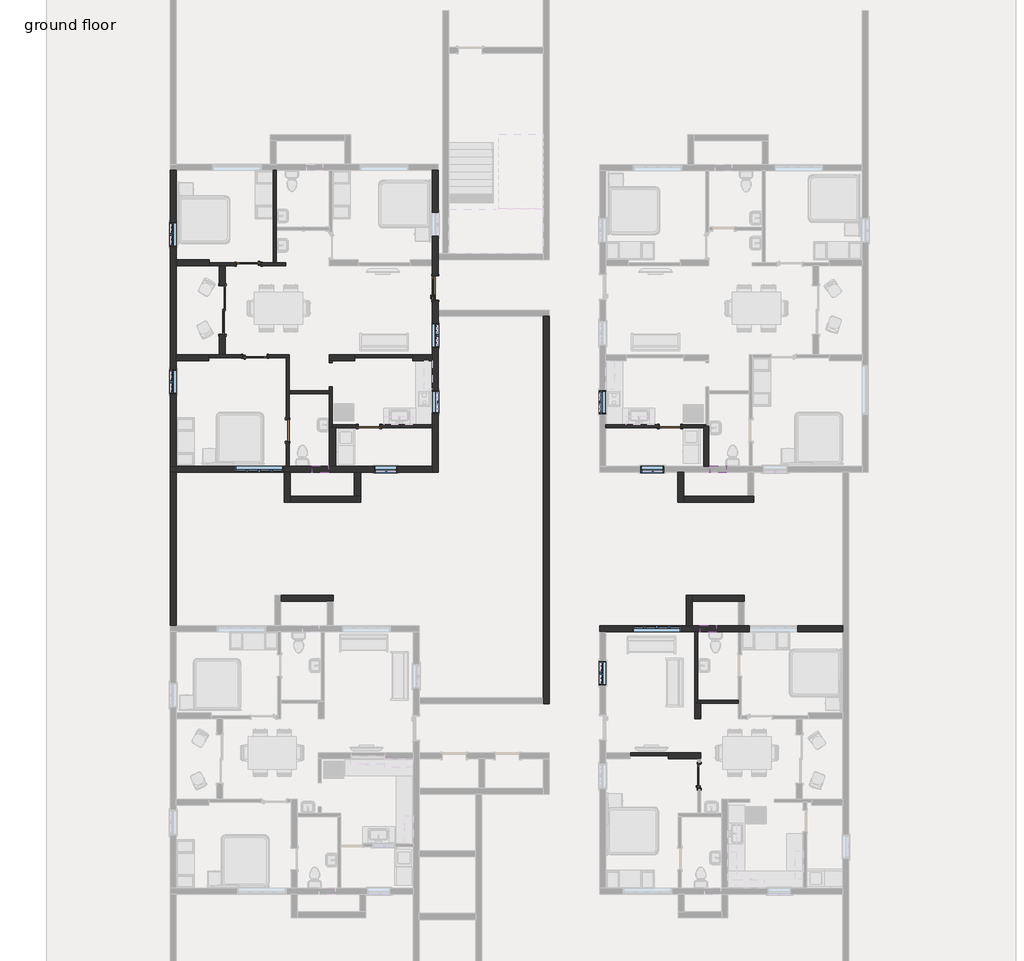
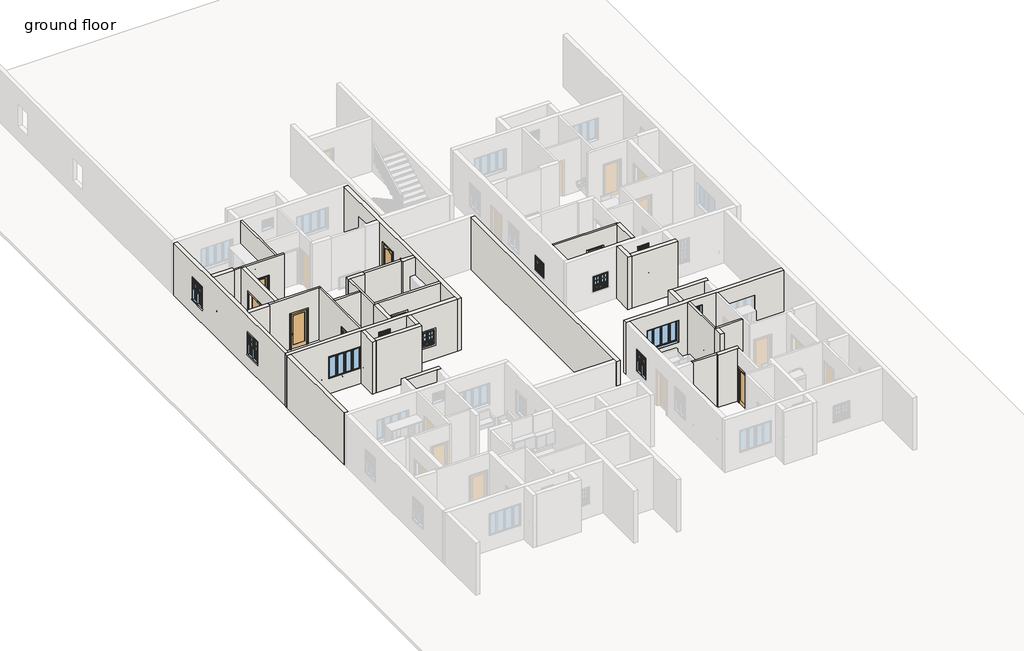
# One storey, part 6 of 16: 36 walls, 13 windows, 8 doors.
"""IFC4 building model written with IfcOpenShell, lengths in millimetres."""

from ifc_helpers import new_model, si_unit, point, frame, origin, place, context, project, spatial, polyline, ellipse_curve, trimmed, outline, extrude, faceted_brep, transform, mapped, element, save
from ifc_brep_helpers import plane_surface, extruded_surface, advanced_brep
from components import door_fe8ae985, door_d4d75d1e, door_a3feeac7, door_3c6ab76a, door_38851409, door_d141acb4, window_ced37e8f, window_5487fb6d, window_f2d8fef0, window_45970670

model = new_model("IFC4")

# Units and contexts
model_context = context("Model", 3, world=origin())
ifc_project = project(units=[si_unit("LENGTHUNIT", "METRE", prefix="MILLI")], contexts=[model_context])

# Site, building, storey
site = spatial("IfcSite", under=ifc_project)
building = spatial("IfcBuilding", under=site)
storey = spatial("IfcBuildingStorey", under=building, Name="ground floor", Elevation=609.6)

# Doors
placement = place(None, origin())
door_shape = door_fe8ae985(model_context)
element("IfcDoor", 1, ObjectType="36\" x 84\"", at=placement, inside=storey, context=model_context, shape_type="MappedRepresentation", body=[
    mapped(door_shape, transform((53146.051243, 27978.3344264, 609.6), x_axis=(0.0, -1.0, 0.0), y_axis=(1.0, 0.0, 0.0), z_axis=(0.0, 0.0, 1.0))),
])
door_2_shape = door_d4d75d1e(model_context)
element("IfcDoor", 2, ObjectType="Door-Double-Sliding : 72\" x 84\"", at=placement, inside=storey, context=model_context, shape_type="MappedRepresentation", body=[
    mapped(door_2_shape, transform((44983.126243, 27148.9150652, 609.6), x_axis=(0.0, -1.0, 0.0), y_axis=(1.0, 0.0, 0.0), z_axis=(0.0, 0.0, 1.0))),
])
door_3_shape = door_a3feeac7(model_context)
element("IfcDoor", 3, ObjectType="Door-Interior-Single-1_Panel-Wood : 36\" x 84\"", at=placement, inside=storey, context=model_context, shape_type="MappedRepresentation", body=[
    mapped(door_3_shape, transform((46097.551243, 28879.2900652, 609.6), x_axis=(-1.0, 0.0, 0.0), y_axis=(0.0, -1.0, 0.0), z_axis=(0.0, 0.0, 1.0))),
])
element("IfcDoor", 4, ObjectType="Door-Interior-Single-1_Panel-Wood : 36\" x 84\"", at=placement, inside=storey, context=model_context, shape_type="MappedRepresentation", body=[
    mapped(door_3_shape, transform((46338.851243, 25405.8400652, 609.6), x_axis=(1.0, 0.0, 0.0), y_axis=(0.0, 1.0, 0.0), z_axis=(0.0, 0.0, 1.0))),
])
door_4_shape = door_3c6ab76a(model_context)
element("IfcDoor", 5, ObjectType="Door-Interior-Single-1_Panel-Wood : 36\" x 84\"", at=placement, inside=storey, context=model_context, shape_type="MappedRepresentation", body=[
    mapped(door_4_shape, transform((63106.2062819, 9553.0650652, 609.6), x_axis=(0.0, 1.0, 0.0), y_axis=(-1.0, 0.0, 0.0), z_axis=(0.0, 0.0, 1.0))),
])
door_5_shape = door_38851409(model_context)
element("IfcDoor", 6, ObjectType="Single-Flush : 32\" x 84\"", at=placement, inside=storey, context=model_context, shape_type="MappedRepresentation", body=[
    mapped(door_5_shape, transform((47567.576243, 22592.7211333, 609.6), x_axis=(0.0, 1.0, 0.0), y_axis=(-1.0, 0.0, 0.0), z_axis=(0.0, 0.0, 1.0))),
])
element("IfcDoor", 7, ObjectType="Single-Flush : 32\" x 84\"", at=placement, inside=storey, context=model_context, shape_type="MappedRepresentation", body=[
    mapped(door_5_shape, transform((61998.1312819, 22754.7150652, 609.6), x_axis=(1.0, 0.0, 0.0), y_axis=(0.0, 1.0, 0.0), z_axis=(0.0, 0.0, 1.0))),
])
door_6_shape = door_d141acb4(model_context)
element("IfcDoor", 8, ObjectType="Single-Flush : 32\" x 84\"", at=placement, inside=storey, context=model_context, shape_type="MappedRepresentation", body=[
    mapped(door_6_shape, transform((50634.626243, 22754.7150652, 609.6), x_axis=(-1.0, 0.0, 0.0), y_axis=(0.0, -1.0, 0.0), z_axis=(0.0, 0.0, 1.0))),
])

# Walls
element("IfcWall", 9, ObjectType="Generic - 4.5\"", at=placement, inside=storey, context=model_context, shape_type="Brep", body=[
    faceted_brep([(62404.5312819, 22697.5650652, 2743.2), (62404.5312819, 22697.5650652, 609.6), (63268.1312819, 22697.5650652, 609.6), (63268.1312819, 22697.5650652, 3810.0), (59585.1312819, 22697.5650652, 3810.0), (59585.1312819, 22697.5650652, 609.6), (61591.7312819, 22697.5650652, 609.6), (61591.7312819, 22697.5650652, 2743.2), (63357.0312819, 22811.8650652, 609.6), (62404.5312819, 22811.8650652, 609.6), (62404.5312819, 22811.8650652, 2743.2), (61591.7312819, 22811.8650652, 2743.2), (61591.7312819, 22811.8650652, 609.6), (59585.1312819, 22811.8650652, 609.6), (59585.1312819, 22811.8650652, 3810.0), (63357.0312819, 22811.8650652, 3810.0), (63357.0312819, 22754.7150652, 609.6), (63268.1312819, 22754.7150652, 609.6), (63268.1312819, 22754.7150652, 3810.0), (63357.0312819, 22754.7150652, 3810.0)], [[[0, 1, 2, 3, 4, 5, 6, 7]], [[8, 9, 10, 11, 12, 13, 14, 15]], [[6, 5, 13, 12]], [[2, 1, 9, 8, 16, 17]], [[4, 3, 18, 19, 15, 14]], [[3, 2, 17, 18]], [[17, 16, 19, 18]], [[16, 8, 15, 19]], [[5, 4, 14, 13]], [[10, 9, 1, 0]], [[11, 10, 0, 7]], [[12, 11, 7, 6]]]),
])
element("IfcWall", 10, ObjectType="Generic - 4.5\"", at=placement, inside=storey, context=model_context, shape_type="Brep", body=[
    faceted_brep([(47027.826243, 32412.9272014, 609.6), (47027.826243, 28933.2650652, 609.6), (47027.826243, 28933.2650652, 3810.0), (47027.826243, 32412.9272014, 3810.0), (47142.126243, 32412.9272014, 609.6), (47142.126243, 32412.9272014, 3810.0), (47142.126243, 30266.7650652, 3810.0), (47142.126243, 30152.4650652, 3810.0), (47142.126243, 28933.2650652, 3810.0), (47142.126243, 28933.2650652, 609.6), (47142.126243, 30152.4650652, 609.6), (47142.126243, 30266.7650652, 609.6)], [[[0, 1, 2, 3]], [[4, 5, 6, 7, 8, 9, 10, 11]], [[1, 0, 4, 11, 10, 9]], [[3, 2, 8, 7, 6, 5]], [[0, 3, 5, 4]], [[2, 1, 9, 8]]]),
])
element("IfcWall", 11, ObjectType="Generic - 4.5\"", at=placement, inside=storey, context=model_context, shape_type="Brep", body=[
    faceted_brep([(47027.826243, 32412.9272014, 609.6), (47027.826243, 28933.2650652, 609.6), (47027.826243, 28933.2650652, 3810.0), (47027.826243, 32412.9272014, 3810.0), (47142.126243, 32412.9272014, 609.6), (47142.126243, 32412.9272014, 3810.0), (47142.126243, 30266.7650652, 3810.0), (47142.126243, 30152.4650652, 3810.0), (47142.126243, 28933.2650652, 3810.0), (47142.126243, 28933.2650652, 609.6), (47142.126243, 30152.4650652, 609.6), (47142.126243, 30266.7650652, 609.6)], [[[0, 1, 2, 3]], [[4, 5, 6, 7, 8, 9, 10, 11]], [[1, 0, 4, 11, 10, 9]], [[3, 2, 8, 7, 6, 5]], [[0, 3, 5, 4]], [[2, 1, 9, 8]]]),
])
element("IfcWall", 12, ObjectType="Generic - 4.5\"", at=placement, inside=storey, context=model_context, shape_type="Brep", body=[
    faceted_brep([(47498.5665582, 28818.9650652, 609.6), (47498.5665582, 28818.9650652, 3810.0), (45224.426243, 28818.9650652, 3810.0), (44995.826243, 28818.9650652, 3810.0), (44602.9665582, 28818.9650652, 3810.0), (44602.9665582, 28818.9650652, 609.6), (44995.826243, 28818.9650652, 609.6), (45224.426243, 28818.9650652, 609.6), (45614.951243, 28818.9650652, 609.6), (45614.951243, 28818.9650652, 2768.6), (46580.151243, 28818.9650652, 2768.6), (46580.151243, 28818.9650652, 609.6), (47498.5665582, 28933.2650652, 3810.0), (47498.5665582, 28933.2650652, 609.6), (47142.126243, 28933.2650652, 609.6), (47027.826243, 28933.2650652, 609.6), (46580.151243, 28933.2650652, 609.6), (46580.151243, 28933.2650652, 2768.6), (45614.951243, 28933.2650652, 2768.6), (45614.951243, 28933.2650652, 609.6), (44602.9665582, 28933.2650652, 609.6), (44602.9665582, 28933.2650652, 3810.0), (47027.826243, 28933.2650652, 3810.0), (47142.126243, 28933.2650652, 3810.0)], [[[0, 1, 2, 3, 4, 5, 6, 7, 8, 9, 10, 11]], [[12, 13, 14, 15, 16, 17, 18, 19, 20, 21, 22, 23]], [[13, 0, 11, 16, 15, 14]], [[5, 20, 19, 8, 7, 6]], [[1, 0, 13, 12]], [[4, 3, 2, 1, 12, 23, 22, 21]], [[5, 4, 21, 20]], [[18, 9, 8, 19]], [[9, 18, 17, 10]], [[10, 17, 16, 11]]]),
])
element("IfcWall", 13, ObjectType="Generic - 4.5\"", at=placement, inside=storey, context=model_context, shape_type="Brep", body=[
    faceted_brep([(47624.726243, 25351.8650652, 3810.0), (47510.426243, 25351.8650652, 3810.0), (44588.5228455, 25351.8650652, 3810.0), (44588.5228455, 25351.8650652, 609.6), (45856.251243, 25351.8650652, 609.6), (45856.251243, 25351.8650652, 2768.6), (46821.451243, 25351.8650652, 2768.6), (46821.451243, 25351.8650652, 609.6), (47510.426243, 25351.8650652, 609.6), (47624.726243, 25351.8650652, 609.6), (44588.5228455, 25466.1650652, 3810.0), (44995.826243, 25466.1650652, 3810.0), (45224.426243, 25466.1650652, 3810.0), (47624.726243, 25466.1650652, 3810.0), (47624.726243, 25466.1650652, 609.6), (46821.451243, 25466.1650652, 609.6), (46821.451243, 25466.1650652, 2768.6), (45856.251243, 25466.1650652, 2768.6), (45856.251243, 25466.1650652, 609.6), (45224.426243, 25466.1650652, 609.6), (44995.826243, 25466.1650652, 609.6), (44588.5228455, 25466.1650652, 609.6)], [[[0, 1, 2, 3, 4, 5, 6, 7, 8, 9]], [[10, 11, 12, 13, 14, 15, 16, 17, 18, 19, 20, 21]], [[3, 21, 20, 19, 18, 4]], [[14, 9, 8, 7, 15]], [[2, 1, 0, 13, 12, 11, 10]], [[3, 2, 10, 21]], [[0, 9, 14, 13]], [[6, 16, 15, 7]], [[16, 6, 5, 17]], [[17, 5, 4, 18]]]),
])
element("IfcWall", 14, ObjectType="Generic - 4.5\"", at=placement, inside=storey, context=model_context, shape_type="Brep", body=[
    faceted_brep([(47510.426243, 25351.8650652, 609.6), (47510.426243, 22999.1211333, 609.6), (47510.426243, 22999.1211333, 2743.2), (47510.426243, 22186.3211333, 2743.2), (47510.426243, 22186.3211333, 609.6), (47510.426243, 21249.6272014, 609.6), (47510.426243, 21249.6272014, 3810.0), (47510.426243, 25351.8650652, 3810.0), (47624.726243, 22999.1211333, 2743.2), (47624.726243, 22999.1211333, 609.6), (47624.726243, 23992.9650652, 609.6), (47624.726243, 24107.2650652, 609.6), (47624.726243, 25351.8650652, 609.6), (47624.726243, 25351.8650652, 3810.0), (47624.726243, 24107.2650652, 3810.0), (47624.726243, 23992.9650652, 3810.0), (47624.726243, 21249.6272014, 3810.0), (47624.726243, 21249.6272014, 609.6), (47624.726243, 22186.3211333, 609.6), (47624.726243, 22186.3211333, 2743.2)], [[[0, 1, 2, 3, 4, 5, 6, 7]], [[8, 9, 10, 11, 12, 13, 14, 15, 16, 17, 18, 19]], [[18, 17, 5, 4]], [[12, 11, 10, 9, 1, 0]], [[7, 6, 16, 15, 14, 13]], [[0, 7, 13, 12]], [[6, 5, 17, 16]], [[2, 1, 9, 8]], [[3, 2, 8, 19]], [[4, 3, 19, 18]]]),
])
element("IfcWall", 15, ObjectType="Generic - 4.5\"", at=placement, inside=storey, context=model_context, shape_type="SweptSolid", body=[
    extrude(outline(polyline([(49148.726243, 23992.9650652), (47624.726243, 23992.9650652), (47624.726243, 24107.2650652), (49148.726243, 24107.2650652), (49148.726243, 23992.9650652)])), frame((0.0, 0.0, 609.6), z_axis=(0.0, 0.0, 1.0), x_axis=(1.0, 0.0, 0.0)), (0.0, 0.0, 1.0), 3200.4),
])
element("IfcWall", 16, ObjectType="Generic - 4.5\"", at=placement, inside=storey, context=model_context, shape_type="AdvancedBrep", body=[
    advanced_brep(
    [(49148.726243, 25237.5650652, 609.6), (49148.726243, 25158.1900652, 609.6), (49148.726243, 25158.1900652, 2540.0), (49148.726243, 24243.7900652, 2540.0), (49148.726243, 24243.7900652, 609.6), (49148.726243, 24107.2650652, 609.6), (49148.726243, 23992.9650652, 609.6), (49148.726243, 22697.5650652, 609.6), (49148.726243, 22697.5650652, 3810.0), (49148.726243, 23992.9650652, 3810.0), (49148.726243, 24107.2650652, 3810.0), (49148.726243, 25237.5650652, 3810.0), (49263.026243, 25158.1900652, 2540.0), (49263.026243, 25158.1900652, 609.6), (49263.026243, 25237.5650652, 609.6), (49263.026243, 25237.5650652, 3810.0), (49263.026243, 22811.8650652, 3810.0), (49263.026243, 22697.5650652, 3810.0), (49263.026243, 22697.5650652, 609.6), (49263.026243, 22811.8650652, 609.6), (49263.026243, 24243.7900652, 609.6), (49263.026243, 24243.7900652, 2540.0)],
    [
        (0, 1),
        (1, 2),
        (2, 3, ellipse_curve(frame((49148.726243, 24700.9900652, 2540.0), z_axis=(1.0, 0.0, 0.0), x_axis=(0.0, 1.0, 0.0)), 457.2, 203.2)),
        (3, 4),
        (4, 5),
        (5, 6),
        (6, 7),
        (7, 8),
        (8, 9),
        (9, 10),
        (10, 11),
        (11, 0),
        (12, 13),
        (13, 14),
        (14, 15),
        (15, 16),
        (16, 17),
        (17, 18),
        (18, 19),
        (19, 20),
        (20, 21),
        (21, 12, ellipse_curve(frame((49263.026243, 24700.9900652, 2540.0), z_axis=(-1.0, 0.0, 0.0), x_axis=(0.0, 1.0, 0.0)), 457.2, 203.2)),
        (13, 1),
        (0, 14),
        (18, 7),
        (4, 20),
        (8, 17),
        (15, 11),
        (2, 12),
        (21, 3),
    ],
    [
        plane_surface(frame((49148.726243, 24107.2650652, 609.6), z_axis=(-1.0, 0.0, 0.0), x_axis=(0.0, -1.0, 0.0))),
        plane_surface(frame((49263.026243, 24107.2650652, 609.6), z_axis=(1.0, 0.0, 0.0), x_axis=(0.0, 1.0, 0.0))),
        plane_surface(frame((49148.726243, 25351.8650652, 609.6), z_axis=(0.0, 0.0, -1.0), x_axis=(1.0, 0.0, 0.0))),
        plane_surface(frame((49148.726243, 22754.7150652, 3810.0), z_axis=(0.0, 0.0, 1.0), x_axis=(1.0, 0.0, 0.0))),
        plane_surface(frame((49283.7527857, 22697.5650652, 609.6), z_axis=(0.0, -1.0, 0.0), x_axis=(1.0, 0.0, 0.0))),
        plane_surface(frame((50047.2611034, 25237.5650652, 609.6), z_axis=(0.0, 1.0, 0.0), x_axis=(1.0, 0.0, 0.0))),
        extruded_surface(trimmed(ellipse_curve(frame((49377.326243, 24700.9900652, 2540.0), z_axis=(1.0, 0.0, 0.0), x_axis=(0.0, 1.0, 0.0)), 457.2, 203.2), [point((49377.326243, 25158.1900652, 2540.0))], [point((49377.326243, 24243.7900652, 2540.0))], True, "CARTESIAN"), (-114.30000000000291, 0.0, 0.0), 114.30000000000291),
        plane_surface(frame((49148.726243, 24243.7900652, 2540.0), z_axis=(0.0, 1.0, 0.0), x_axis=(1.0, 0.0, 0.0))),
        plane_surface(frame((49148.726243, 25158.1900652, 609.6), z_axis=(0.0, -1.0, 0.0), x_axis=(1.0, 0.0, 0.0))),
    ],
    [
        (0, [[1, 2, 3, 4, 5, 6, 7, 8, 9, 10, 11, 12]]),
        (1, [[13, 14, 15, 16, 17, 18, 19, 20, 21, 22]]),
        (2, [[-14, 23, -1, 24]]),
        (2, [[-20, -19, 25, -7, -6, -5, 26]]),
        (3, [[-11, -10, -9, 27, -17, -16, 28]]),
        (4, [[-8, -25, -18, -27]]),
        (5, [[-12, -28, -15, -24]]),
        (6, [[-3, 29, -22, 30]]),
        (7, [[-4, -30, -21, -26]]),
        (8, [[-2, -23, -13, -29]]),
    ],
),
])
element("IfcWall", 17, ObjectType="Generic - 4.5\"", at=placement, inside=storey, context=model_context, shape_type="Brep", body=[
    faceted_brep([(49263.026243, 22697.5650652, 609.6), (49377.326243, 22697.5650652, 609.6), (50228.226243, 22697.5650652, 609.6), (50228.226243, 22697.5650652, 2743.2), (51041.026243, 22697.5650652, 2743.2), (51041.026243, 22697.5650652, 609.6), (53034.926243, 22697.5650652, 609.6), (53034.926243, 22697.5650652, 3810.0), (49377.326243, 22697.5650652, 3810.0), (49263.026243, 22697.5650652, 3810.0), (50228.226243, 22811.8650652, 2743.2), (50228.226243, 22811.8650652, 609.6), (49263.026243, 22811.8650652, 609.6), (49263.026243, 22811.8650652, 3810.0), (53034.926243, 22811.8650652, 3810.0), (53034.926243, 22811.8650652, 609.6), (51041.026243, 22811.8650652, 609.6), (51041.026243, 22811.8650652, 2743.2)], [[[0, 1, 2, 3, 4, 5, 6, 7, 8, 9]], [[10, 11, 12, 13, 14, 15, 16, 17]], [[16, 15, 6, 5]], [[12, 11, 2, 1, 0]], [[9, 8, 7, 14, 13]], [[0, 9, 13, 12]], [[7, 6, 15, 14]], [[3, 2, 11, 10]], [[4, 3, 10, 17]], [[5, 4, 17, 16]]]),
])
element("IfcWall", 18, ObjectType="Generic - 4.5\"", at=placement, inside=storey, context=model_context, shape_type="SweptSolid", body=[
    extrude(outline(polyline([(52298.326243, 25351.8650652), (50101.226243, 25351.8650652), (50101.226243, 25466.1650652), (52298.326243, 25466.1650652), (52298.326243, 25351.8650652)])), frame((0.0, 0.0, 609.6), z_axis=(0.0, 0.0, 1.0), x_axis=(1.0, 0.0, 0.0)), (0.0, 0.0, 1.0), 3200.4),
])
element("IfcWall", 19, ObjectType="Generic - 4.5\"", at=placement, inside=storey, context=model_context, shape_type="Brep", body=[
    faceted_brep([(62937.9312819, 15001.3650652, 609.6), (62937.9312819, 12296.2650652, 609.6), (62937.9312819, 12296.2650652, 3810.0), (62937.9312819, 15001.3650652, 3810.0), (63052.2312819, 15001.3650652, 609.6), (63052.2312819, 15001.3650652, 3810.0), (63052.2312819, 12410.5650652, 3810.0), (63052.2312819, 12296.2650652, 3810.0), (63052.2312819, 12296.2650652, 609.6), (63052.2312819, 12410.5650652, 609.6)], [[[0, 1, 2, 3]], [[4, 5, 6, 7, 8, 9]], [[1, 0, 4, 9, 8]], [[3, 2, 7, 6, 5]], [[0, 3, 5, 4]], [[2, 1, 8, 7]]]),
])
element("IfcWall", 20, ObjectType="Generic - 4.5\"", at=placement, inside=storey, context=model_context, shape_type="Brep", body=[
    faceted_brep([(63052.2312819, 12296.2650652, 609.6), (63166.5312819, 12296.2650652, 609.6), (64576.2312819, 12296.2650652, 609.6), (64576.2312819, 12296.2650652, 3810.0), (63166.5312819, 12296.2650652, 3810.0), (63052.2312819, 12296.2650652, 3810.0), (63052.2312819, 12410.5650652, 609.6), (63052.2312819, 12410.5650652, 3810.0), (64576.2312819, 12410.5650652, 3810.0), (64576.2312819, 12410.5650652, 609.6)], [[[0, 1, 2, 3, 4, 5]], [[6, 7, 8, 9]], [[2, 1, 0, 6, 9]], [[5, 4, 3, 8, 7]], [[0, 5, 7, 6]], [[3, 2, 9, 8]]]),
])
element("IfcWall", 21, ObjectType="Generic - 4.5\"", at=placement, inside=storey, context=model_context, shape_type="SweptSolid", body=[
    extrude(outline(polyline([(61941.6438292, 10315.0650652), (60499.5312819, 10315.0650652), (60499.5312819, 10429.3650652), (61941.6438292, 10429.3650652), (61941.6438292, 10315.0650652)])), frame((0.0, 0.0, 609.6), z_axis=(0.0, 0.0, 1.0), x_axis=(1.0, 0.0, 0.0)), (0.0, 0.0, 1.0), 3200.4),
])
element("IfcWall", 22, ObjectType="Generic - 8\"", at=placement, inside=storey, context=model_context, shape_type="Brep", body=[
    faceted_brep([(63471.3312819, 21249.7650652, 609.6), (63471.3312819, 22754.7150652, 609.6), (63471.3312819, 22754.7150652, 3810.0), (63471.3312819, 21249.7650652, 3810.0), (63268.1312819, 21249.7650652, 609.6), (63268.1312819, 21249.7650652, 3810.0), (63268.1312819, 22697.5650652, 3810.0), (63268.1312819, 22754.7150652, 3810.0), (63268.1312819, 22754.7150652, 609.6), (63268.1312819, 22697.5650652, 609.6), (63357.0312819, 22754.7150652, 609.6), (63357.0312819, 22754.7150652, 3810.0)], [[[0, 1, 2, 3]], [[4, 5, 6, 7, 8, 9]], [[1, 0, 4, 9, 8, 10]], [[2, 1, 10, 8, 7, 11]], [[3, 2, 11, 7, 6, 5]], [[0, 3, 5, 4]]]),
])
element("IfcWall", 23, ObjectType="Generic - 9\"", at=placement, inside=storey, context=model_context, shape_type="Brep", body=[
    faceted_brep([(62290.2312819, 21021.1650652, 609.6), (62290.2312819, 19895.3539393, 609.6), (62290.2312819, 19895.3539393, 3810.0), (62290.2312819, 21021.1650652, 3810.0), (62518.8312819, 21021.1650652, 609.6), (62518.8312819, 21021.1650652, 3810.0), (62518.8312819, 20123.9539393, 3810.0), (62518.8312819, 19895.3539393, 3810.0), (62518.8312819, 19895.3539393, 609.6), (62518.8312819, 20123.9539393, 609.6)], [[[0, 1, 2, 3]], [[4, 5, 6, 7, 8, 9]], [[1, 0, 4, 9, 8]], [[3, 2, 7, 6, 5]], [[0, 3, 5, 4]], [[2, 1, 8, 7]]]),
])
element("IfcWall", 24, ObjectType="Generic - 9\"", at=placement, inside=storey, context=model_context, shape_type="Brep", body=[
    faceted_brep([(62518.8312819, 19895.3539393, 609.6), (65172.2983059, 19895.3539393, 609.6), (65172.2983059, 19895.3539393, 3810.0), (62518.8312819, 19895.3539393, 3810.0), (62518.8312819, 20123.9539393, 609.6), (62518.8312819, 20123.9539393, 3810.0), (64943.6983059, 20123.9539393, 3810.0), (65172.2983059, 20123.9539393, 3810.0), (65172.2983059, 20123.9539393, 609.6), (64943.6983059, 20123.9539393, 609.6)], [[[0, 1, 2, 3]], [[4, 5, 6, 7, 8, 9]], [[1, 0, 4, 9, 8]], [[3, 2, 7, 6, 5]], [[0, 3, 5, 4]], [[2, 1, 8, 7]]]),
])
element("IfcWall", 25, ObjectType="Generic - 9\"", at=placement, inside=storey, context=model_context, shape_type="Brep", body=[
    faceted_brep([(53034.926243, 21021.0272014, 3810.0), (53034.926243, 21249.6272014, 3810.0), (53034.926243, 22697.5650652, 3810.0), (53034.926243, 22811.8650652, 3810.0), (53034.926243, 25237.5650652, 3810.0), (53034.926243, 25466.1650652, 3810.0), (53034.926243, 28818.9650652, 3810.0), (53034.926243, 29047.5650652, 3810.0), (53034.926243, 32412.9272014, 3810.0), (53034.926243, 32412.9272014, 609.6), (53034.926243, 29047.5650652, 609.6), (53034.926243, 28818.9650652, 609.6), (53034.926243, 28460.9344264, 609.6), (53034.926243, 28460.9344264, 2768.6), (53034.926243, 27495.7344264, 2768.6), (53034.926243, 27495.7344264, 609.6), (53034.926243, 25466.1650652, 609.6), (53034.926243, 25237.5650652, 609.6), (53034.926243, 22811.8650652, 609.6), (53034.926243, 22697.5650652, 609.6), (53034.926243, 21249.6272014, 609.6), (53034.926243, 21021.0272014, 609.6), (53034.926243, 26644.8344264, 2844.8), (53034.926243, 25730.4344264, 2844.8), (53034.926243, 25730.4344264, 1524.0), (53034.926243, 26644.8344264, 1524.0), (53034.926243, 30838.2650652, 2844.8), (53034.926243, 29923.8650652, 2844.8), (53034.926243, 29923.8650652, 1524.0), (53034.926243, 30838.2650652, 1524.0), (53034.926243, 23240.4900652, 2438.4), (53034.926243, 23240.4900652, 1524.0), (53034.926243, 24104.0900652, 1524.0), (53034.926243, 24104.0900652, 2438.4), (53263.526243, 32412.9272014, 3810.0), (53263.526243, 29276.1650652, 3810.0), (53263.526243, 29047.5650652, 3810.0), (53263.526243, 27137.7037877, 3810.0), (53263.526243, 26909.1037877, 3810.0), (53263.526243, 21021.0272014, 3810.0), (53263.526243, 21021.0272014, 609.6), (53263.526243, 26909.1037877, 609.6), (53263.526243, 27137.7037877, 609.6), (53263.526243, 27495.7344264, 609.6), (53263.526243, 27495.7344264, 2768.6), (53263.526243, 28460.9344264, 2768.6), (53263.526243, 28460.9344264, 609.6), (53263.526243, 29047.5650652, 609.6), (53263.526243, 29276.1650652, 609.6), (53263.526243, 32412.9272014, 609.6), (53263.526243, 26644.8344264, 2844.8), (53263.526243, 26644.8344264, 1524.0), (53263.526243, 25730.4344264, 1524.0), (53263.526243, 25730.4344264, 2844.8), (53263.526243, 30838.2650652, 2844.8), (53263.526243, 30838.2650652, 1524.0), (53263.526243, 29923.8650652, 1524.0), (53263.526243, 29923.8650652, 2844.8), (53263.526243, 23240.4900652, 2438.4), (53263.526243, 24104.0900652, 2438.4), (53263.526243, 24104.0900652, 1524.0), (53263.526243, 23240.4900652, 1524.0)], [[[0, 1, 2, 3, 4, 5, 6, 7, 8, 9, 10, 11, 12, 13, 14, 15, 16, 17, 18, 19, 20, 21], [22, 23, 24, 25], [26, 27, 28, 29], [30, 31, 32, 33]], [[34, 35, 36, 37, 38, 39, 40, 41, 42, 43, 44, 45, 46, 47, 48, 49], [50, 51, 52, 53], [54, 55, 56, 57], [58, 59, 60, 61]], [[9, 49, 48, 47, 46, 12, 11, 10]], [[40, 21, 20, 19, 18, 17, 16, 15, 43, 42, 41]], [[8, 7, 6, 5, 4, 3, 2, 1, 0, 39, 38, 37, 36, 35, 34]], [[9, 8, 34, 49]], [[0, 21, 40, 39]], [[14, 44, 43, 15]], [[44, 14, 13, 45]], [[45, 13, 12, 46]], [[51, 50, 22, 25]], [[52, 51, 25, 24]], [[53, 52, 24, 23]], [[50, 53, 23, 22]], [[55, 54, 26, 29]], [[56, 55, 29, 28]], [[57, 56, 28, 27]], [[54, 57, 27, 26]], [[31, 30, 58, 61]], [[32, 31, 61, 60]], [[33, 32, 60, 59]], [[30, 33, 59, 58]]]),
])
element("IfcWall", 26, ObjectType="Generic - 9\"", at=placement, inside=storey, context=model_context, shape_type="Brep", body=[
    faceted_brep([(53034.926243, 21249.6272014, 609.6), (49377.326243, 21249.6272014, 609.6), (49148.726243, 21249.6272014, 609.6), (47624.726243, 21249.6272014, 609.6), (47510.426243, 21249.6272014, 609.6), (43370.226243, 21249.6272014, 609.6), (43141.626243, 21249.6272014, 609.6), (43141.626243, 21249.6272014, 3810.0), (43370.226243, 21249.6272014, 3810.0), (47510.426243, 21249.6272014, 3810.0), (47624.726243, 21249.6272014, 3810.0), (49148.726243, 21249.6272014, 3810.0), (49377.326243, 21249.6272014, 3810.0), (53034.926243, 21249.6272014, 3810.0), (45580.859219, 21249.6272014, 2870.2), (45580.859219, 21249.6272014, 1524.0), (47409.659219, 21249.6272014, 1524.0), (47409.659219, 21249.6272014, 2870.2), (50843.18, 21249.6272014, 2438.4), (50843.18, 21249.6272014, 1524.0), (51706.78, 21249.6272014, 1524.0), (51706.78, 21249.6272014, 2438.4), (49110.626243, 21249.6272014, 3352.8), (48501.026243, 21249.6272014, 3352.8), (48501.026243, 21249.6272014, 2743.2), (49110.626243, 21249.6272014, 2743.2), (53034.926243, 21021.0272014, 609.6), (53034.926243, 21021.0272014, 3810.0), (50322.48, 21021.0272014, 3810.0), (50093.88, 21021.0272014, 3810.0), (47676.359219, 21021.0272014, 3810.0), (47447.759219, 21021.0272014, 3810.0), (43370.226243, 21021.0272014, 3810.0), (43141.626243, 21021.0272014, 3810.0), (43141.626243, 21021.0272014, 609.6), (43370.226243, 21021.0272014, 609.6), (47447.759219, 21021.0272014, 609.6), (47676.359219, 21021.0272014, 609.6), (50093.88, 21021.0272014, 609.6), (50322.48, 21021.0272014, 609.6), (45580.859219, 21021.0272014, 2870.2), (47409.659219, 21021.0272014, 2870.2), (47409.659219, 21021.0272014, 1524.0), (45580.859219, 21021.0272014, 1524.0), (50843.18, 21021.0272014, 2438.4), (51706.78, 21021.0272014, 2438.4), (51706.78, 21021.0272014, 1524.0), (50843.18, 21021.0272014, 1524.0), (49110.626243, 21021.0272014, 3352.8), (49110.626243, 21021.0272014, 2743.2), (48501.026243, 21021.0272014, 2743.2), (48501.026243, 21021.0272014, 3352.8)], [[[0, 1, 2, 3, 4, 5, 6, 7, 8, 9, 10, 11, 12, 13], [14, 15, 16, 17], [18, 19, 20, 21], [22, 23, 24, 25]], [[26, 27, 28, 29, 30, 31, 32, 33, 34, 35, 36, 37, 38, 39], [40, 41, 42, 43], [44, 45, 46, 47], [48, 49, 50, 51]], [[6, 5, 4, 3, 2, 1, 0, 26, 39, 38, 37, 36, 35, 34]], [[13, 12, 11, 10, 9, 8, 7, 33, 32, 31, 30, 29, 28, 27]], [[0, 13, 27, 26]], [[7, 6, 34, 33]], [[15, 14, 40, 43]], [[16, 15, 43, 42]], [[17, 16, 42, 41]], [[14, 17, 41, 40]], [[19, 18, 44, 47]], [[20, 19, 47, 46]], [[21, 20, 46, 45]], [[18, 21, 45, 44]], [[49, 48, 22, 25]], [[50, 49, 25, 24]], [[51, 50, 24, 23]], [[48, 51, 23, 22]]]),
])
element("IfcWall", 27, ObjectType="Generic - 9\"", at=placement, inside=storey, context=model_context, shape_type="Brep", body=[
    faceted_brep([(43370.226243, 21249.6272014, 609.6), (43370.226243, 25237.5650652, 609.6), (43370.226243, 25466.1650652, 609.6), (43370.226243, 28818.9650652, 609.6), (43370.226243, 29047.5650652, 609.6), (43370.226243, 32412.9272014, 609.6), (43370.226243, 32412.9272014, 3810.0), (43370.226243, 29047.5650652, 3810.0), (43370.226243, 28818.9650652, 3810.0), (43370.226243, 25466.1650652, 3810.0), (43370.226243, 25237.5650652, 3810.0), (43370.226243, 21249.6272014, 3810.0), (43370.226243, 23980.2650652, 2844.8), (43370.226243, 24894.6650652, 2844.8), (43370.226243, 24894.6650652, 1524.0), (43370.226243, 23980.2650652, 1524.0), (43370.226243, 29542.8650652, 2844.8), (43370.226243, 30457.2650652, 2844.8), (43370.226243, 30457.2650652, 1524.0), (43370.226243, 29542.8650652, 1524.0), (43141.626243, 21249.6272014, 609.6), (43141.626243, 21249.6272014, 3810.0), (43141.626243, 32412.9272014, 3810.0), (43141.626243, 32412.9272014, 609.6), (43141.626243, 23980.2650652, 2844.8), (43141.626243, 23980.2650652, 1524.0), (43141.626243, 24894.6650652, 1524.0), (43141.626243, 24894.6650652, 2844.8), (43141.626243, 29542.8650652, 2844.8), (43141.626243, 29542.8650652, 1524.0), (43141.626243, 30457.2650652, 1524.0), (43141.626243, 30457.2650652, 2844.8)], [[[0, 1, 2, 3, 4, 5, 6, 7, 8, 9, 10, 11], [12, 13, 14, 15], [16, 17, 18, 19]], [[20, 21, 22, 23], [24, 25, 26, 27], [28, 29, 30, 31]], [[5, 4, 3, 2, 1, 0, 20, 23]], [[11, 10, 9, 8, 7, 6, 22, 21]], [[0, 11, 21, 20]], [[6, 5, 23, 22]], [[25, 24, 12, 15]], [[26, 25, 15, 14]], [[27, 26, 14, 13]], [[24, 27, 13, 12]], [[29, 28, 16, 19]], [[30, 29, 19, 18]], [[31, 30, 18, 17]], [[28, 31, 17, 16]]]),
])
element("IfcWall", 28, ObjectType="Generic - 9\"", at=placement, inside=storey, context=model_context, shape_type="Brep", body=[
    faceted_brep([(43370.226243, 28818.9650652, 609.6), (44602.9665582, 28818.9650652, 609.6), (44602.9665582, 28818.9650652, 3810.0), (43370.226243, 28818.9650652, 3810.0), (43370.226243, 29047.5650652, 609.6), (43370.226243, 29047.5650652, 3810.0), (44602.9665582, 29047.5650652, 3810.0), (44602.9665582, 29047.5650652, 609.6), (44602.9665582, 28933.2650652, 609.6), (44602.9665582, 28933.2650652, 3810.0)], [[[0, 1, 2, 3]], [[4, 5, 6, 7]], [[1, 0, 4, 7, 8]], [[2, 1, 8, 7, 6, 9]], [[3, 2, 9, 6, 5]], [[0, 3, 5, 4]]]),
])
element("IfcWall", 29, ObjectType="Generic - 9\"", at=placement, inside=storey, context=model_context, shape_type="SweptSolid", body=[
    extrude(outline(polyline([(26234.5150652, 2743.2), (26234.5150652, 609.6), (25466.1650652, 609.6), (25466.1650652, 3810.0), (28818.9650652, 3810.0), (28818.9650652, 609.6), (28063.3150652, 609.6), (28063.3150652, 2743.2), (26234.5150652, 2743.2)])), frame((44995.826243, 0.0, 0.0), z_axis=(1.0, 0.0, 0.0), x_axis=(0.0, 1.0, 0.0)), (0.0, 0.0, 1.0), 228.6),
])
element("IfcWall", 30, ObjectType="Generic - 9\"", at=placement, inside=storey, context=model_context, shape_type="Brep", body=[
    faceted_brep([(43370.226243, 25237.5650652, 609.6), (44588.5228455, 25237.5650652, 609.6), (44588.5228455, 25237.5650652, 3810.0), (43370.226243, 25237.5650652, 3810.0), (43370.226243, 25466.1650652, 609.6), (43370.226243, 25466.1650652, 3810.0), (44588.5228455, 25466.1650652, 3810.0), (44588.5228455, 25466.1650652, 609.6), (44588.5228455, 25351.8650652, 609.6), (44588.5228455, 25351.8650652, 3810.0)], [[[0, 1, 2, 3]], [[4, 5, 6, 7]], [[1, 0, 4, 7, 8]], [[2, 1, 8, 7, 6, 9]], [[3, 2, 9, 6, 5]], [[0, 3, 5, 4]]]),
])
element("IfcWall", 31, ObjectType="Generic - 9\"", at=placement, inside=storey, context=model_context, shape_type="Brep", body=[
    faceted_brep([(49377.326243, 21249.6272014, 609.6), (49377.326243, 22697.5650652, 609.6), (49377.326243, 22697.5650652, 3810.0), (49377.326243, 21249.6272014, 3810.0), (49148.726243, 21249.6272014, 609.6), (49148.726243, 21249.6272014, 3810.0), (49148.726243, 22697.5650652, 3810.0), (49148.726243, 22697.5650652, 609.6), (49263.026243, 22697.5650652, 609.6), (49263.026243, 22697.5650652, 3810.0)], [[[0, 1, 2, 3]], [[4, 5, 6, 7]], [[1, 0, 4, 7, 8]], [[3, 2, 9, 6, 5]], [[0, 3, 5, 4]], [[2, 1, 8, 7, 6, 9]]]),
])
element("IfcWall", 32, ObjectType="Generic - 9\"", at=placement, inside=storey, context=model_context, shape_type="Brep", body=[
    faceted_brep([(53034.926243, 25466.1650652, 609.6), (52298.326243, 25466.1650652, 609.6), (52298.326243, 25466.1650652, 3810.0), (53034.926243, 25466.1650652, 3810.0), (53034.926243, 25237.5650652, 609.6), (53034.926243, 25237.5650652, 3810.0), (52298.326243, 25237.5650652, 3810.0), (52298.326243, 25237.5650652, 609.6), (52298.326243, 25351.8650652, 609.6), (52298.326243, 25351.8650652, 3810.0)], [[[0, 1, 2, 3]], [[4, 5, 6, 7]], [[1, 0, 4, 7, 8]], [[2, 1, 8, 7, 6, 9]], [[3, 2, 9, 6, 5]], [[0, 3, 5, 4]]]),
])
element("IfcWall", 33, ObjectType="Generic - 9\"", at=placement, inside=storey, context=model_context, shape_type="Brep", body=[
    faceted_brep([(50101.226243, 25466.1650652, 609.6), (49148.726243, 25466.1650652, 609.6), (49148.726243, 25466.1650652, 3810.0), (50101.226243, 25466.1650652, 3810.0), (50101.226243, 25237.5650652, 609.6), (50101.226243, 25237.5650652, 3810.0), (49263.026243, 25237.5650652, 3810.0), (49148.726243, 25237.5650652, 3810.0), (49148.726243, 25237.5650652, 609.6), (49263.026243, 25237.5650652, 609.6), (50101.226243, 25351.8650652, 609.6), (50101.226243, 25351.8650652, 3810.0)], [[[0, 1, 2, 3]], [[4, 5, 6, 7, 8, 9]], [[1, 0, 10, 4, 9, 8]], [[3, 2, 7, 6, 5, 11]], [[0, 3, 11, 5, 4, 10]], [[2, 1, 8, 7]]]),
])
element("IfcWall", 34, ObjectType="Generic - 9\"", at=placement, inside=storey, context=model_context, shape_type="Brep", body=[
    faceted_brep([(47447.759219, 21021.0272014, 609.6), (47447.759219, 19895.3539393, 609.6), (47447.759219, 19895.3539393, 3810.0), (47447.759219, 21021.0272014, 3810.0), (47676.359219, 21021.0272014, 609.6), (47676.359219, 21021.0272014, 3810.0), (47676.359219, 20123.9539393, 3810.0), (47676.359219, 19895.3539393, 3810.0), (47676.359219, 19895.3539393, 609.6), (47676.359219, 20123.9539393, 609.6)], [[[0, 1, 2, 3]], [[4, 5, 6, 7, 8, 9]], [[1, 0, 4, 9, 8]], [[3, 2, 7, 6, 5]], [[0, 3, 5, 4]], [[2, 1, 8, 7]]]),
])
element("IfcWall", 35, ObjectType="Generic - 9\"", at=placement, inside=storey, context=model_context, shape_type="Brep", body=[
    faceted_brep([(47676.359219, 19895.3539393, 609.6), (50322.48, 19895.3539393, 609.6), (50322.48, 19895.3539393, 3810.0), (47676.359219, 19895.3539393, 3810.0), (47676.359219, 20123.9539393, 609.6), (47676.359219, 20123.9539393, 3810.0), (50093.88, 20123.9539393, 3810.0), (50322.48, 20123.9539393, 3810.0), (50322.48, 20123.9539393, 609.6), (50093.88, 20123.9539393, 609.6)], [[[0, 1, 2, 3]], [[4, 5, 6, 7, 8, 9]], [[1, 0, 4, 9, 8]], [[3, 2, 7, 6, 5]], [[0, 3, 5, 4]], [[2, 1, 8, 7]]]),
])
element("IfcWall", 36, ObjectType="Generic - 9\"", at=placement, inside=storey, context=model_context, shape_type="SweptSolid", body=[
    extrude(outline(polyline([(50322.48, 21021.0272014), (50322.48, 20123.9539393), (50093.88, 20123.9539393), (50093.88, 21021.0272014), (50322.48, 21021.0272014)])), frame((0.0, 0.0, 609.6), z_axis=(0.0, 0.0, 1.0), x_axis=(1.0, 0.0, 0.0)), (0.0, 0.0, 1.0), 3200.4),
])
element("IfcWall", 37, ObjectType="Generic - 9\"", at=placement, inside=storey, context=model_context, shape_type="Brep", body=[
    faceted_brep([(47319.926243, 16147.8755101, 609.6), (49056.9877548, 16147.8755101, 609.6), (49285.5877548, 16147.8755101, 609.6), (49285.5877548, 16147.8755101, 3810.0), (49056.9877548, 16147.8755101, 3810.0), (47319.926243, 16147.8755101, 3810.0), (47319.926243, 16376.4755101, 609.6), (47319.926243, 16376.4755101, 3810.0), (49285.5877548, 16376.4755101, 3810.0), (49285.5877548, 16376.4755101, 609.6)], [[[0, 1, 2, 3, 4, 5]], [[6, 7, 8, 9]], [[2, 1, 0, 6, 9]], [[5, 4, 3, 8, 7]], [[0, 5, 7, 6]], [[3, 2, 9, 8]]]),
])
element("IfcWall", 38, ObjectType="Generic - 9\"", at=placement, inside=storey, context=model_context, shape_type="Brep", body=[
    faceted_brep([(59356.5312819, 15001.3650652, 609.6), (59585.1312819, 15001.3650652, 609.6), (62937.9312819, 15001.3650652, 609.6), (63052.2312819, 15001.3650652, 609.6), (64576.2312819, 15001.3650652, 609.6), (64690.5312819, 15001.3650652, 609.6), (68525.9312819, 15001.3650652, 609.6), (68525.9312819, 15001.3650652, 3810.0), (64690.5312819, 15001.3650652, 3810.0), (64576.2312819, 15001.3650652, 3810.0), (63052.2312819, 15001.3650652, 3810.0), (62937.9312819, 15001.3650652, 3810.0), (59585.1312819, 15001.3650652, 3810.0), (59356.5312819, 15001.3650652, 3810.0), (66824.1312819, 15001.3650652, 2870.2), (66824.1312819, 15001.3650652, 1524.0), (64995.3312819, 15001.3650652, 1524.0), (64995.3312819, 15001.3650652, 2870.2), (62420.06977, 15001.3650652, 2870.2), (62420.06977, 15001.3650652, 1524.0), (60591.26977, 15001.3650652, 1524.0), (60591.26977, 15001.3650652, 2870.2), (63147.4812819, 15001.3650652, 3352.8), (63757.0812819, 15001.3650652, 3352.8), (63757.0812819, 15001.3650652, 2743.2), (63147.4812819, 15001.3650652, 2743.2), (59356.5312819, 15229.9650652, 609.6), (59356.5312819, 15229.9650652, 3810.0), (62610.56977, 15229.9650652, 3810.0), (62839.16977, 15229.9650652, 3810.0), (64576.2312819, 15229.9650652, 3810.0), (64804.8312819, 15229.9650652, 3810.0), (68525.9312819, 15229.9650652, 3810.0), (68525.9312819, 15229.9650652, 609.6), (64804.8312819, 15229.9650652, 609.6), (64576.2312819, 15229.9650652, 609.6), (62839.16977, 15229.9650652, 609.6), (62610.56977, 15229.9650652, 609.6), (66824.1312819, 15229.9650652, 2870.2), (64995.3312819, 15229.9650652, 2870.2), (64995.3312819, 15229.9650652, 1524.0), (66824.1312819, 15229.9650652, 1524.0), (62420.06977, 15229.9650652, 2870.2), (60591.26977, 15229.9650652, 2870.2), (60591.26977, 15229.9650652, 1524.0), (62420.06977, 15229.9650652, 1524.0), (63147.4812819, 15229.9650652, 3352.8), (63147.4812819, 15229.9650652, 2743.2), (63757.0812819, 15229.9650652, 2743.2), (63757.0812819, 15229.9650652, 3352.8)], [[[0, 1, 2, 3, 4, 5, 6, 7, 8, 9, 10, 11, 12, 13], [14, 15, 16, 17], [18, 19, 20, 21], [22, 23, 24, 25]], [[26, 27, 28, 29, 30, 31, 32, 33, 34, 35, 36, 37], [38, 39, 40, 41], [42, 43, 44, 45], [46, 47, 48, 49]], [[6, 5, 4, 3, 2, 1, 0, 26, 37, 36, 35, 34, 33]], [[13, 12, 11, 10, 9, 8, 7, 32, 31, 30, 29, 28, 27]], [[7, 6, 33, 32]], [[0, 13, 27, 26]], [[15, 14, 38, 41]], [[16, 15, 41, 40]], [[17, 16, 40, 39]], [[14, 17, 39, 38]], [[19, 18, 42, 45]], [[20, 19, 45, 44]], [[21, 20, 44, 43]], [[18, 21, 43, 42]], [[47, 46, 22, 25]], [[48, 47, 25, 24]], [[49, 48, 24, 23]], [[46, 49, 23, 22]]]),
])
element("IfcWall", 39, ObjectType="Generic - 9\"", at=placement, inside=storey, context=model_context, shape_type="Brep", body=[
    faceted_brep([(61941.6438292, 10200.7650652, 609.6), (63052.2312819, 10200.7650652, 609.6), (63166.5312819, 10200.7650652, 609.6), (63166.5312819, 10200.7650652, 3810.0), (63052.2312819, 10200.7650652, 3810.0), (61941.6438292, 10200.7650652, 3810.0), (61941.6438292, 10429.3650652, 609.6), (61941.6438292, 10429.3650652, 3810.0), (63166.5312819, 10429.3650652, 3810.0), (63166.5312819, 10429.3650652, 609.6), (61941.6438292, 10315.0650652, 609.6), (61941.6438292, 10315.0650652, 3810.0)], [[[0, 1, 2, 3, 4, 5]], [[6, 7, 8, 9]], [[2, 1, 0, 10, 6, 9]], [[5, 4, 3, 8, 7, 11]], [[0, 5, 11, 7, 6, 10]], [[3, 2, 9, 8]]]),
])
element("IfcWall", 40, ObjectType="Generic - 9\"", at=placement, inside=storey, context=model_context, shape_type="Brep", body=[
    faceted_brep([(63166.5312819, 11724.7650652, 609.6), (63166.5312819, 12296.2650652, 609.6), (63166.5312819, 12296.2650652, 3810.0), (63166.5312819, 11724.7650652, 3810.0), (62937.9312819, 11724.7650652, 609.6), (62937.9312819, 11724.7650652, 3810.0), (62937.9312819, 12296.2650652, 3810.0), (62937.9312819, 12296.2650652, 609.6), (63052.2312819, 12296.2650652, 609.6), (63052.2312819, 12296.2650652, 3810.0)], [[[0, 1, 2, 3]], [[4, 5, 6, 7]], [[1, 0, 4, 7, 8]], [[3, 2, 9, 6, 5]], [[0, 3, 5, 4]], [[2, 1, 8, 7, 6, 9]]]),
])
element("IfcWall", 41, ObjectType="Generic - 9\"", at=placement, inside=storey, context=model_context, shape_type="Brep", body=[
    faceted_brep([(62839.16977, 15229.9650652, 609.6), (62839.16977, 16147.8755101, 609.6), (62839.16977, 16376.4755101, 609.6), (62839.16977, 16376.4755101, 3810.0), (62839.16977, 16147.8755101, 3810.0), (62839.16977, 15229.9650652, 3810.0), (62610.56977, 15229.9650652, 609.6), (62610.56977, 15229.9650652, 3810.0), (62610.56977, 16376.4755101, 3810.0), (62610.56977, 16376.4755101, 609.6)], [[[0, 1, 2, 3, 4, 5]], [[6, 7, 8, 9]], [[2, 1, 0, 6, 9]], [[5, 4, 3, 8, 7]], [[0, 5, 7, 6]], [[3, 2, 9, 8]]]),
])
element("IfcWall", 42, ObjectType="Generic - 9\"", at=placement, inside=storey, context=model_context, shape_type="Brep", body=[
    faceted_brep([(62839.16977, 16147.8755101, 609.6), (64576.2312819, 16147.8755101, 609.6), (64804.8312819, 16147.8755101, 609.6), (64804.8312819, 16147.8755101, 3810.0), (64576.2312819, 16147.8755101, 3810.0), (62839.16977, 16147.8755101, 3810.0), (62839.16977, 16376.4755101, 609.6), (62839.16977, 16376.4755101, 3810.0), (64804.8312819, 16376.4755101, 3810.0), (64804.8312819, 16376.4755101, 609.6)], [[[0, 1, 2, 3, 4, 5]], [[6, 7, 8, 9]], [[2, 1, 0, 6, 9]], [[5, 4, 3, 8, 7]], [[0, 5, 7, 6]], [[3, 2, 9, 8]]]),
])
element("IfcWall", 43, ObjectType="Generic - 9\"", at=placement, inside=storey, context=model_context, shape_type="Brep", body=[
    faceted_brep([(57222.9312819, 26909.1037877, 609.6), (57222.9312819, 12518.2417893, 609.6), (57222.9312819, 12289.6417893, 609.6), (57222.9312819, 12289.6417893, 3810.0), (57222.9312819, 12518.2417893, 3810.0), (57222.9312819, 26909.1037877, 3810.0), (57451.5312819, 26909.1037877, 609.6), (57451.5312819, 26909.1037877, 3810.0), (57451.5312819, 12289.6417893, 3810.0), (57451.5312819, 12289.6417893, 609.6)], [[[0, 1, 2, 3, 4, 5]], [[6, 7, 8, 9]], [[2, 1, 0, 6, 9]], [[5, 4, 3, 8, 7]], [[0, 5, 7, 6]], [[3, 2, 9, 8]]]),
])
element("IfcWall", 44, ObjectType="Generic - 9\"", at=placement, inside=storey, context=model_context, shape_type="SweptSolid", body=[
    extrude(outline(polyline([(43141.626243, 15226.6718163), (43141.626243, 21021.0272014), (43370.226243, 21021.0272014), (43370.226243, 15226.6718163), (43141.626243, 15226.6718163)])), frame((0.0, 0.0, 609.6), z_axis=(0.0, 0.0, 1.0), x_axis=(1.0, 0.0, 0.0)), (0.0, 0.0, 1.0), 3200.4),
])

# Windows
window_shape = window_ced37e8f(model_context)
element("IfcWindow", 45, ObjectType="Window-Casement-Double-Awning : 34\" x 36\"", at=placement, inside=storey, context=model_context, shape_type="MappedRepresentation", body=[
    mapped(window_shape, transform((59470.8312819, 23669.1150652, 609.6), x_axis=(0.0, 1.0, 0.0), y_axis=(-1.0, 0.0, 0.0), z_axis=(0.0, 0.0, 1.0))),
])
element("IfcWindow", 46, ObjectType="Window-Casement-Double-Awning : 34\" x 36\"", at=placement, inside=storey, context=model_context, shape_type="MappedRepresentation", body=[
    mapped(window_shape, transform((61337.7312819, 21135.4650652, 609.6), x_axis=(-1.0, 0.0, 0.0), y_axis=(0.0, -1.0, 0.0), z_axis=(0.0, 0.0, 1.0))),
])
element("IfcWindow", 47, ObjectType="Window-Casement-Double-Awning : 34\" x 36\"", at=placement, inside=storey, context=model_context, shape_type="MappedRepresentation", body=[
    mapped(window_shape, transform((51274.98, 21135.3272014, 609.6), x_axis=(-1.0, 0.0, 0.0), y_axis=(0.0, -1.0, 0.0), z_axis=(0.0, 0.0, 1.0))),
])
element("IfcWindow", 48, ObjectType="Window-Casement-Double-Awning : 34\" x 36\"", at=placement, inside=storey, context=model_context, shape_type="MappedRepresentation", body=[
    mapped(window_shape, transform((53149.226243, 23672.2900652, 609.6), x_axis=(0.0, -1.0, 0.0), y_axis=(1.0, 0.0, 0.0), z_axis=(0.0, 0.0, 1.0))),
])
window_2_shape = window_5487fb6d(model_context)
element("IfcWindow", 49, ObjectType="Window-Casement-Multi-Sash-Horizontal : 72\" x 53\"", at=placement, inside=storey, context=model_context, shape_type="MappedRepresentation", body=[
    mapped(window_2_shape, transform((61505.66977, 15115.6650652, 609.6), x_axis=(1.0, 0.0, 0.0), y_axis=(0.0, 1.0, 0.0), z_axis=(0.0, 0.0, 1.0))),
])
element("IfcWindow", 50, ObjectType="Window-Casement-Multi-Sash-Horizontal : 72\" x 53\"", at=placement, inside=storey, context=model_context, shape_type="MappedRepresentation", body=[
    mapped(window_2_shape, transform((46495.259219, 21135.3272014, 609.6), x_axis=(-1.0, 0.0, 0.0), y_axis=(0.0, -1.0, 0.0), z_axis=(0.0, 0.0, 1.0))),
])
window_3_shape = window_f2d8fef0(model_context)
element("IfcWindow", 51, ObjectType="Window-Louvers : 24\" x 24\"", at=placement, inside=storey, context=model_context, shape_type="MappedRepresentation", body=[
    mapped(window_3_shape, transform((63826.9312819, 21129.1150652, 1828.8), x_axis=(-1.0, 0.0, 0.0), y_axis=(0.0, -1.0, 0.0), z_axis=(0.0, 0.0, 1.0))),
])
element("IfcWindow", 52, ObjectType="Window-Louvers : 24\" x 24\"", at=placement, inside=storey, context=model_context, shape_type="MappedRepresentation", body=[
    mapped(window_3_shape, transform((63452.2812819, 15122.0150652, 1828.8), x_axis=(1.0, 0.0, 0.0), y_axis=(0.0, 1.0, 0.0), z_axis=(0.0, 0.0, 1.0))),
])
element("IfcWindow", 53, ObjectType="Window-Louvers : 24\" x 24\"", at=placement, inside=storey, context=model_context, shape_type="MappedRepresentation", body=[
    mapped(window_3_shape, transform((48805.826243, 21128.9772014, 1828.8), x_axis=(-1.0, 0.0, 0.0), y_axis=(0.0, -1.0, 0.0), z_axis=(0.0, 0.0, 1.0))),
])
window_4_shape = window_45970670(model_context)
element("IfcWindow", 54, ObjectType="Window-Single-Hung-Double : 36\" x 52\"", at=placement, inside=storey, context=model_context, shape_type="MappedRepresentation", body=[
    mapped(window_4_shape, transform((59470.8312819, 13439.2650652, 609.6), x_axis=(0.0, 1.0, 0.0), y_axis=(-1.0, 0.0, 0.0), z_axis=(0.0, 0.0, 1.0))),
])
element("IfcWindow", 55, ObjectType="Window-Single-Hung-Double : 36\" x 52\"", at=placement, inside=storey, context=model_context, shape_type="MappedRepresentation", body=[
    mapped(window_4_shape, transform((43255.926243, 24437.4650652, 609.6), x_axis=(0.0, 1.0, 0.0), y_axis=(-1.0, 0.0, 0.0), z_axis=(0.0, 0.0, 1.0))),
])
element("IfcWindow", 56, ObjectType="Window-Single-Hung-Double : 36\" x 52\"", at=placement, inside=storey, context=model_context, shape_type="MappedRepresentation", body=[
    mapped(window_4_shape, transform((53149.226243, 26187.6344264, 609.6), x_axis=(0.0, -1.0, 0.0), y_axis=(1.0, 0.0, 0.0), z_axis=(0.0, 0.0, 1.0))),
])
element("IfcWindow", 57, ObjectType="Window-Single-Hung-Double : 36\" x 52\"", at=placement, inside=storey, context=model_context, shape_type="MappedRepresentation", body=[
    mapped(window_4_shape, transform((43255.926243, 30000.0650652, 609.6), x_axis=(0.0, 1.0, 0.0), y_axis=(-1.0, 0.0, 0.0), z_axis=(0.0, 0.0, 1.0))),
])

save(model, "model.ifc")

# Revit data of these elements
# Type "36\" x 84\""
#   Type Mark = "11"
#   Assembly Code = "B2030100"
#   Analytic Construction = "French door, wood frame with single glass"
#   Threshold Offset [instance default] = 0' - 0 1/2"
#   Thickness = 0' - 1 3/8"
#   Thermal Resistance (R) = 1.0696 (h·ft²·°F)/BTU
#   Swing Angle [instance default] = 90.00°
#   Stiles = 0' - 4 3/4"
#   Rough Width = 3' - 2"
#   Rough Height = 7' - 1"
#   Radius = 1' - 8.05625"
#   Lock Rail = 0' - 7 1/8"
#   Height = 7' - 0"
#   Width = 3' - 0"
#   Heat Transfer Coefficient (U) = 0.9350 BTU/(h·ft²·°F)
#   Door Offset [instance default] = 0' - 0"
#   Bottom Rail = 0' - 9 1/2"
#   Threshold [instance default] = yes
#   Function = 1
#   Exterior Trim [instance default] = yes
#   Trim Material = Cherry
#   Threshold Material = Cherry
#   Panel Material = Cherry
#   Glazing = Glass
#   Frame Material = Cherry
#   Door Handle Material = Aluminum
#   Visual Light Transmittance = 0
#   Solar Heat Gain Coefficient = 0
#   Wall Closure = (empty or 0)
#   Construction Type = (empty or 0)
# Type "Door-Double-Sliding : 72\" x 84\""
#   Type Mark = "12"
#   Construction Type Id = "opn-d45"
#   Assembly Code = "C1020"
#   Analytic Construction = "Wood frame, double glass door "
#   Thickness = 0' - 2"
#   Thermal Resistance (R) = 1.8150 (h·ft²·°F)/BTU
#   Heat Transfer Coefficient (U) = 0.5510 BTU/(h·ft²·°F)
#   Height = 7' - 0"
#   Rail Width = 0' - 2"
#   Stiles = 0' - 2"
#   Trim Projection Ext = 0' - 1"
#   Trim Projection Int = 0' - 1"
#   Trim Width = 0' - 3"
#   Width = 6' - 0"
#   Define Thermal Properties by = 1
#   Glazing = Glass
#   Panel Material = Wood - Birch - Solid Stained Light Low Gloss
#   Trim Material = Paint - Sienna
#   Visual Light Transmittance = 0
#   Solar Heat Gain Coefficient = 0
#   Function = (empty or 0)
#   Wall Closure = (empty or 0)
# Type "Door-Interior-Single-1_Panel-Wood : 36\" x 84\""
#   Type Mark = "8"
#   Assembly Code = "C1020300"
#   Analytic Construction = "Wooden"
#   Top Rail = 0' - 4 11/16"
#   Thickness = 0' - 1 3/8"
#   Thermal Resistance (R) = 2.5876 (h·ft²·°F)/BTU
#   Swing Angle [instance default] = 90.00°
#   Stiles = 0' - 4 3/4"
#   Rough Width = 3' - 2"
#   Rough Height = 7' - 1"
#   Height = 7' - 0"
#   Width = 3' - 0"
#   Heat Transfer Coefficient (U) = 0.3865 BTU/(h·ft²·°F)
#   Bottom Rail = 0' - 9 1/8"
#   Trim Material = Cherry
#   Panel Material = Cherry
#   Frame Material = Cherry
#   Door Handle Material = Aluminum
#   Visual Light Transmittance = 0
#   Solar Heat Gain Coefficient = 0
#   Wall Closure = (empty or 0)
#   Function = (empty or 0)
# Type "Single-Flush : 32\" x 84\""
#   Type Mark = "3"
#   Construction Type Id = "MDOOR"
#   Assembly Code = "C1020"
#   Analytic Construction = "Metal"
#   Thickness = 0' - 2"
#   Heat Transfer Coefficient (U) = 0.651978 BTU/(h·ft²·°F)
#   Height = 7' - 0"
#   Trim Projection Ext = 0' - 1"
#   Trim Projection Int = 0' - 1"
#   Trim Width = 0' - 3"
#   Width = 2' - 8"
#   Define Thermal Properties by = 1
#   Define Thermal Properties by = 1
#   Door Material = Door - Panel
#   Frame Material = Door - Frame
#   Visual Light Transmittance = 0
#   Solar Heat Gain Coefficient = 0
#   Function = (empty or 0)
#   Wall Closure = (empty or 0)
# Type "Generic - 4.5\""
#   Assembly Code = "B2010"
#   Layers, outside or top first: 0' - 4 1/2" no material (function 1)
# Type "Generic - 8\""
#   Assembly Code = "B2010"
#   Layers, outside or top first: 0' - 8" no material (function 1)
# Type "Generic - 9\""
#   Assembly Code = "B2010"
#   Layers, outside or top first: 0' - 9" no material (function 1)
# Type "Window-Casement-Double-Awning : 34\" x 36\""
#   Type Mark = "28"
#   Fire Rating = "0.5h"
#   Assembly Code = "B2020100"
#   Analytic Construction = "Double glazing - domestic"
#   Window Inset [instance default] = 0' - 0"
#   Wall Thickness [instance default] = 0' - 6"
#   Interior Wall Closure [instance default] = 0' - 2 1/4"
#   Half Width = 1' - 5"
#   Visual Light Transmittance = 0.81
#   Thermal Resistance (R) = 1.8146 (h·ft²·°F)/BTU
#   Solar Heat Gain Coefficient = 0.76
#   Rough Width = 2' - 10 1/2"
#   Rough Height = 3' - 0 1/2"
#   Open Window Height = 2' - 0"
#   Height = 3' - 0"
#   Heat Transfer Coefficient (U) = 0.5511 BTU/(h·ft²·°F)
#   Frame Extension [instance default] = 0' - 0 1/4"
#   Exterior Wall Closure [instance default] = 0' - 1 1/4"
#   Awning Height = 1' - 0"
#   Extension Jamb [instance default] = 0' - 2 1/4"
#   Default Sill Height = 3' - 0"
#   Width = 2' - 10"
#   Top Muntin Visibility = yes
#   Interior Trim Visibility [instance default] = yes
#   Bottom Muntin Visibility = yes
#   Exterior Trim Visibility [instance default] = yes
#   Extension Jamb Visibility [instance default] = yes
#   Interior Trim Material = Wood - Stained
#   Muntin Pattern = Muntin Pattern_2x2 : Muntin Pattern_2x2
#   Interior Trim = Trim-Window-Interior-Flat : Picture Frame
#   Interior Frame Material = Wood - Stained
#   Exterior Trim Material = Clad - White
#   Glass Panel Material = Glass
#   Exterior Trim = Trim-Window-Exterior-Flat : with Sill
#   Exterior Frame Material = Clad - White
#   Wall Closure = (empty or 0)
# Type "Window-Casement-Multi-Sash-Horizontal : 72\" x 53\""
#   Type Mark = "24"
#   Fire Rating = "0.5h"
#   Assembly Code = "B2020100"
#   Analytic Construction = "Double glazing - domestic"
#   Window Inset [instance default] = 0' - 0 5/8"
#   Wall Thickness [instance default] = 0' - 6"
#   Visual Light Transmittance = 0.81
#   Thermal Resistance (R) = 1.8146 (h·ft²·°F)/BTU
#   Solar Heat Gain Coefficient = 0.76
#   Rough Width = 6' - 0 1/2"
#   Rough Height = 4' - 5 1/2"
#   Open Window Width = 1' - 6"
#   Heat Transfer Coefficient (U) = 0.5511 BTU/(h·ft²·°F)
#   Height = 4' - 5"
#   Frame Gap 3 [instance default] = 0' - 1 83/128"
#   Frame Gap 2 [instance default] = 0' - 0 5/8"
#   Frame Gap 1 = 0' - 1 51/128"
#   Default Sill Height = 3' - 0"
#   Width = 6' - 0"
#   Frame Material = Metal - Aluminum
#   Glass Panel Material = Glass
#   Wall Closure = (empty or 0)
# Type "Window-Louvers : 24\" x 24\""
#   Type Mark = "18"
#   Construction Type Id = "GSP4R"
#   Assembly Code = "B20"
#   Analytic Construction = "1/8 in Pilkington single glazing"
#   Visual Light Transmittance = 0.9
#   Thermal Resistance (R) = 1.53941 (h·ft²·°F)/BTU
#   Solar Heat Gain Coefficient = 0.78
#   Max Height = 1' - 11.74264"
#   Height = 2' - 0"
#   Heat Transfer Coefficient (U) = 0.6496 BTU/(h·ft²·°F)
#   Blade Width [instance default] = 1' - 10 1/2"
#   Blade Vertical Thickness = 0' - 0.35355"
#   Blade Thickness = 0' - 0 1/4"
#   Blade Spacing = 0' - 1 1/2"
#   Blade Height = 0' - 1.85355"
#   Blade Depth = 0' - 3"
#   Blade Angle = 45.00°
#   Default Sill Height = 3' - 0"
#   Trim Projection_Exterior = 0' - 0 1/2"
#   Trim Projection_Interior = 0' - 0 1/2"
#   Trim Width_Exterior = 0' - 1 1/2"
#   Trim Width_Interior = 0' - 1 1/2"
#   Width = 2' - 0"
#   Max Blade Count = 12
#   Define Thermal Properties by = 1
#   Blade Count = 12
#   Frame Material = Birch
#   Louver Material = Birch
#   Trim Exterior Material = Birch
#   Trim Interior Material = Birch
#   Wall Closure = (empty or 0)
# Type "Window-Single-Hung-Double : 36\" x 52\""
#   Type Mark = "27"
#   Fire Rating = "0.5h"
#   Construction Type Id = "DG-DR"
#   Assembly Code = "B2020100"
#   Analytic Construction = "Double glazing - domestic"
#   Wall Thickness [instance default] = 0' - 6"
#   Window Inset [instance default] = 0' - 0"
#   Visual Light Transmittance = 0.81
#   Thermal Resistance (R) = 1.8146 (h·ft²·°F)/BTU
#   Solar Heat Gain Coefficient = 0.76
#   Muntin Width = 1' - 0 1/16"
#   Muntin Height = 1' - 10 1/8"
#   Interior Wall Closure [instance default] = 0' - 1 1/2"
#   Rough Width = 3' - 0 1/2"
#   Rough Height = 4' - 4 1/2"
#   Frame Extension [instance default] = 0' - 1 1/4"
#   Exterior Wall Closure [instance default] = 0' - 0 1/2"
#   Extension Jamb [instance default] = 0' - 1 1/2"
#   Heat Transfer Coefficient (U) = 0.5511 BTU/(h·ft²·°F)
#   Height = 4' - 4"
#   Width = 3' - 0"
#   Top Muntin Visibility = yes
#   Indicator Visibility [instance default] = yes
#   Extension Jamb Visibility [instance default] = yes
#   Interior Trim Visibility [instance default] = yes
